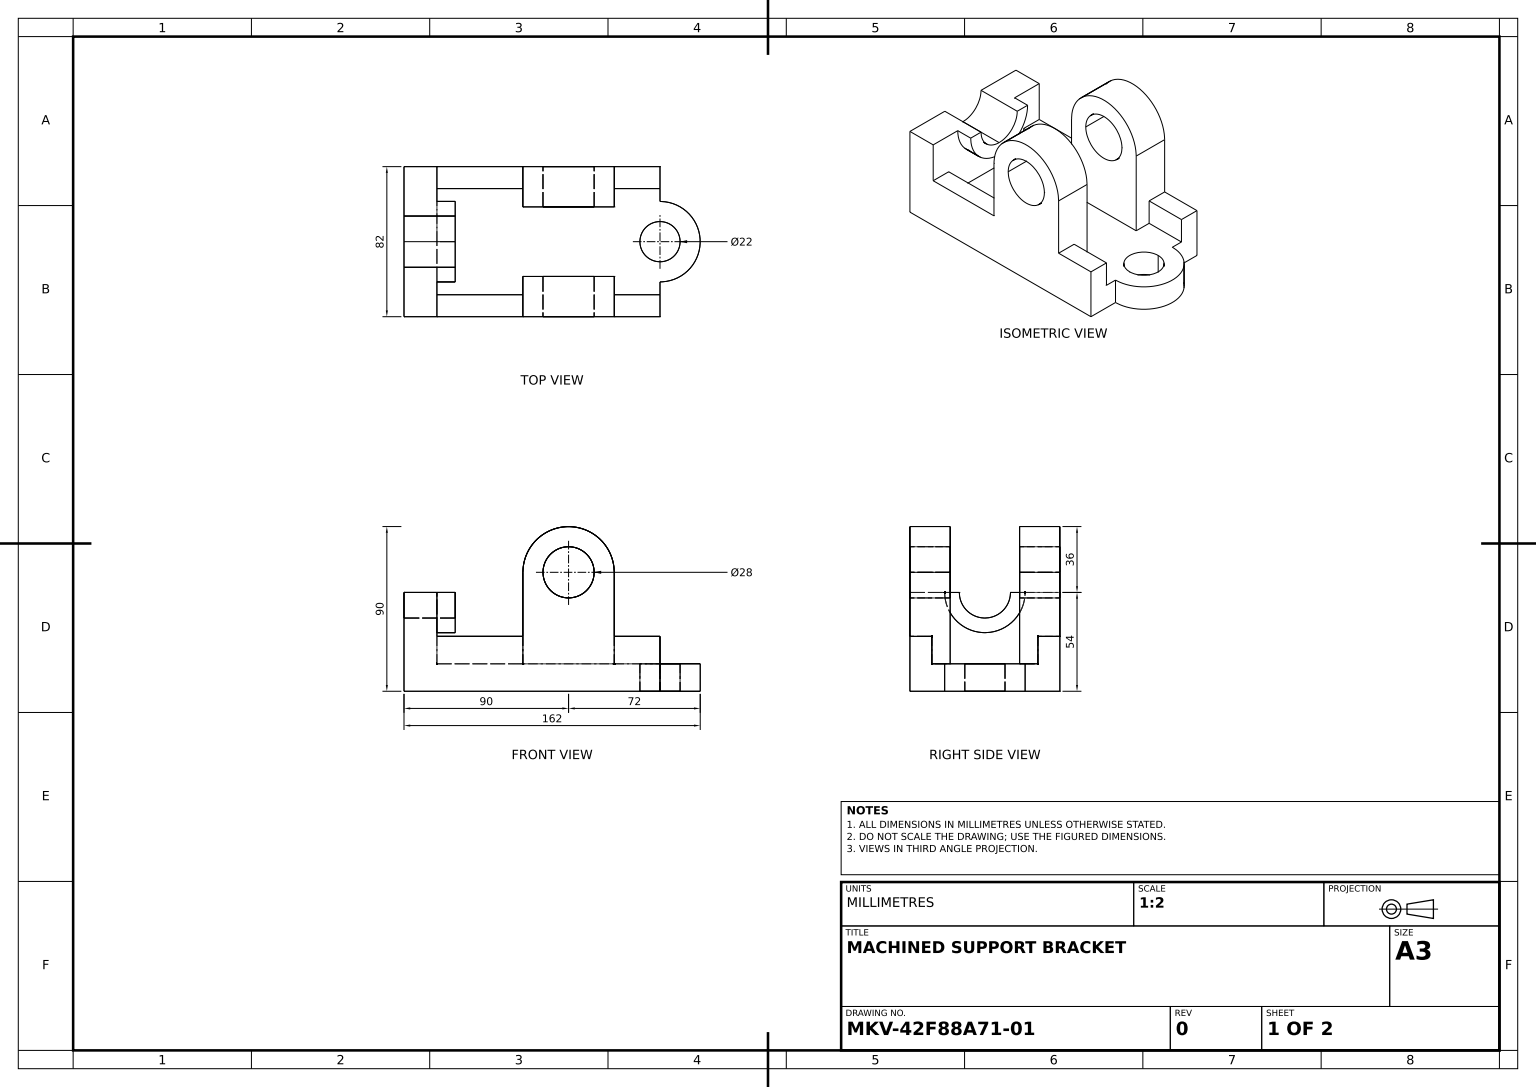
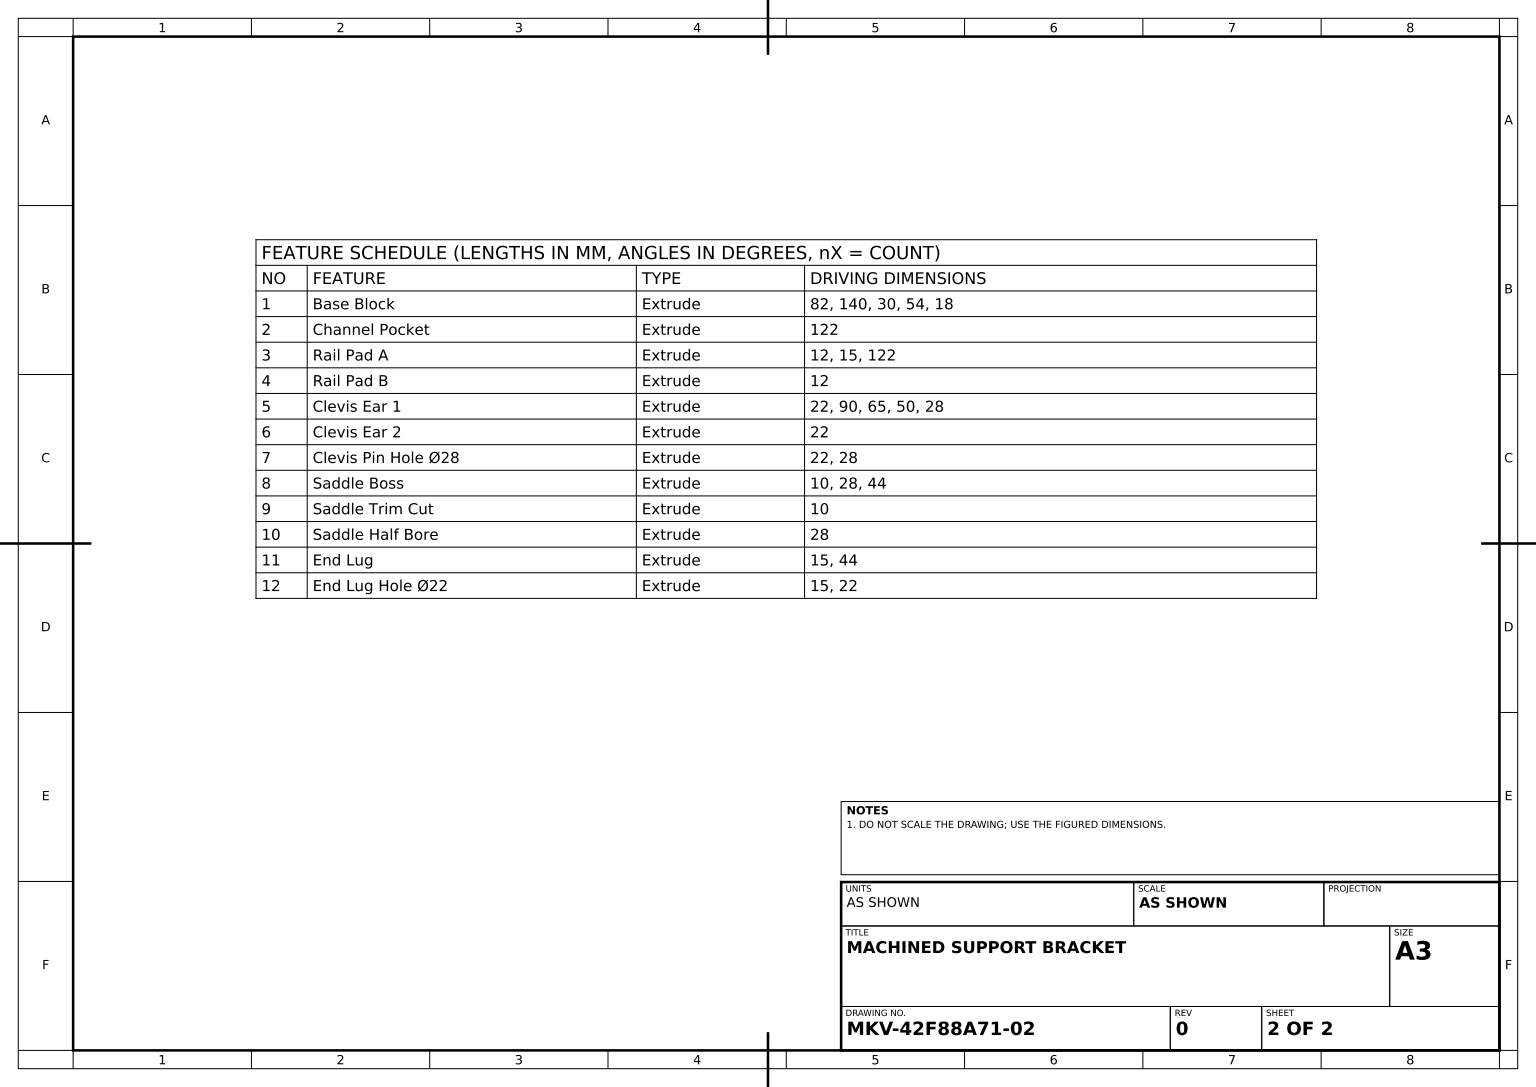
SolidWorks part; units mm, degrees
material "Plain Carbon Steel"
ref_plane "Front Plane" through (0, 0, 0) normal (0, 0, 1) x (1, 0, 0)
ref_plane "Top Plane" through (0, 0, 0) normal (0, 1, 0) x (1, 0, 0)
ref_plane "Right Plane" through (0, 0, 0) normal (1, 0, 0) x (0, 0, -1)
sketch "Base Profile Sketch" plane through (0, 0, 0) normal (0, 0, 1) x (1, 0, 0)
  line L0 (0, 0) -> (0, 54)
  line L1 (0, 54) -> (18, 54)
  line L2 (18, 54) -> (18, 30)
  line L3 (18, 30) -> (140, 30)
  line L4 (140, 30) -> (140, 0)
  line L5 (140, 0) -> (0, 0)
  dimension "D1" = 140
  dimension "D2" = 30
  dimension "D3" = 54
  dimension "D4" = 18
extrude "Base Block" add sketch "Base Profile Sketch" along normal mid plane 82
sketch "Channel Pocket Sketch" plane through (140, 0, 0) normal (1, 0, 0) x (0, 0, -1)
  line L0 (41, 0) -> (41, 30) construction
  line L1 (-41, 30) -> (41, 30)
  line L2 (-41, 30) -> (-41, 15)
  line L3 (-41, 15) -> (41, 15)
  line L4 (41, 30) -> (41, 15)
extrude "Channel Pocket" cut sketch "Channel Pocket Sketch" against normal blind 122
sketch "Rail Pad A Sketch" plane through (0, 0, 41) normal (0, 0, 1) x (1, 0, 0)
  line L1 (18, 15) -> (140, 15)
  line L2 (18, 15) -> (18, 30)
  line L3 (18, 30) -> (140, 30)
  line L4 (140, 15) -> (140, 30)
  dimension "D1" = 15
  dimension "D2" = 122
extrude "Rail Pad A" add sketch "Rail Pad A Sketch" against normal blind 12
sketch "Rail Pad B Sketch" plane through (0, 0, -41) normal (0, 0, -1) x (-1, 0, 0)
  line L1 (-140, 15) -> (-18, 15)
  line L2 (-140, 15) -> (-140, 30)
  line L3 (-140, 30) -> (-18, 30)
  line L4 (-18, 15) -> (-18, 30)
extrude "Rail Pad B" add sketch "Rail Pad B Sketch" against normal blind 12
sketch "Clevis Ear 1 Sketch" plane through (0, 0, 41) normal (0, 0, 1) x (1, 0, 0)
  line L0 (0, 0) -> (90, 0)
  line L1 (0, 0) -> (140, 0) construction
  line L2 (90, 0) -> (90, 65)
  line L3 (65, 65) -> (65, 15)
  line L4 (65, 15) -> (115, 15)
  line L5 (115, 15) -> (115, 65)
  arc A0 (115, 65) -> (65, 65) centre (90, 65) ccw
  circle A1 centre (90, 65) radius 14
  dimension "D3" = 50
  dimension "D4" = 28
  dimension "D1" = 90
  dimension "D2" = 65
  dimension "D5" = 50
extrude "Clevis Ear 1" add sketch "Clevis Ear 1 Sketch" against normal blind 22
sketch "Clevis Ear 2 Sketch" plane through (0, 0, -41) normal (0, 0, -1) x (-1, 0, 0)
  line L3 (-65, 15) -> (-65, 65)
  line L4 (-115, 65) -> (-115, 15)
  line L5 (-115, 15) -> (-65, 15)
  line L6 (-18, 54) -> (-18, 30)
  line L7 (-18, 30) -> (-140, 30)
  line L8 (-140, 30) -> (-140, 0)
  line L9 (-140, 0) -> (0, 0)
  line L10 (0, 0) -> (0, 54)
  line L11 (0, 54) -> (-18, 54)
  line L12 (-18, 54) -> (-18, 30)
  line L13 (-18, 30) -> (-140, 30)
  line L14 (-140, 30) -> (-140, 0)
  line L15 (-140, 0) -> (0, 0)
  line L16 (0, 0) -> (0, 54)
  line L17 (0, 54) -> (-18, 54)
  line L18 (-65, 15) -> (-65, 65)
  line L19 (-115, 65) -> (-115, 15)
  line L20 (-115, 15) -> (-65, 15)
  arc A1 (-65, 65) -> (-115, 65) centre (-90, 65) ccw
  arc A2 (-65, 65) -> (-115, 65) centre (-90, 65) ccw
  dimension "D1" = 0
  dimension "D2" = 0
extrude "Clevis Ear 2" add sketch "Clevis Ear 2 Sketch" against normal blind 22 contours L18 A2 L19 L13 | L19 L20 L18 L13
sketch "Clevis Pin Hole Sketch" plane through (0, 0, -41) normal (0, 0, -1) x (-1, 0, 0)
  line L0 (-115, 65) -> (-65, 65) construction
  circle A2 centre (-90, 65) radius 14
  dimension "D1" = 28
extrude "Clevis Pin Hole Ø28" cut sketch "Clevis Pin Hole Sketch" against normal blind 22
sketch "Saddle Boss Sketch" plane through (18, 0, 0) normal (1, 0, 0) x (0, 0, -1)
  line L0 (-41, 54) -> (41, 54) construction
  circle A0 centre (0, 54) radius 22
  circle A1 centre (0, 54) radius 14
  dimension "D1" = 28
  dimension "D2" = 44
extrude "Saddle Boss" add sketch "Saddle Boss Sketch" along normal blind 10
sketch "Saddle Trim Sketch" plane through (28, 0, 0) normal (1, 0, 0) x (0, 0, -1)
  line L0 (-22, 54) -> (22, 54)
  circle A0 centre (0, 54) radius 14 construction
  circle A1 centre (0, 54) radius 22
  arc A2 (22, 54) -> (-22, 54) centre (0, 54) ccw
  arc A3 (14, 54) -> (-14, 54) centre (0, 54) ccw
  circle M3 centre (0, 54) radius 22
  circle M4 centre (0, 54) radius 14
  dimension "D1" = 0
extrude "Saddle Trim Cut" cut sketch "Saddle Trim Sketch" against normal blind 10 contours L0 M3 M4
sketch "Saddle Bore Sketch" plane through (28, 0, 0) normal (1, 0, 0) x (0, 0, -1)
  line L0 (-14, 54) -> (14, 54) construction
  circle A0 centre (0, 54) radius 14
  dimension "D1" = 28
extrude "Saddle Half Bore" cut sketch "Saddle Bore Sketch" against normal blind 28
sketch "End Lug Sketch" plane through (0, 0, 0) normal (0, -1, 0) x (1, 0, 0)
  line L0 (140, 41) -> (140, -41) construction
  line L1 (140, 22) -> (140, -22)
  arc A0 (140, -22) -> (140, 22) centre (140, 0) ccw
  dimension "D1" = 44
extrude "End Lug" add sketch "End Lug Sketch" against normal blind 15
sketch "End Lug Hole Sketch" plane through (0, 0, 0) normal (0, -1, 0) x (1, 0, 0)
  line L0 (140, 41) -> (140, -41) construction
  circle A0 centre (140, 0) radius 11
  dimension "D1" = 22
extrude "End Lug Hole Ø22" cut sketch "End Lug Hole Sketch" against normal blind 15
